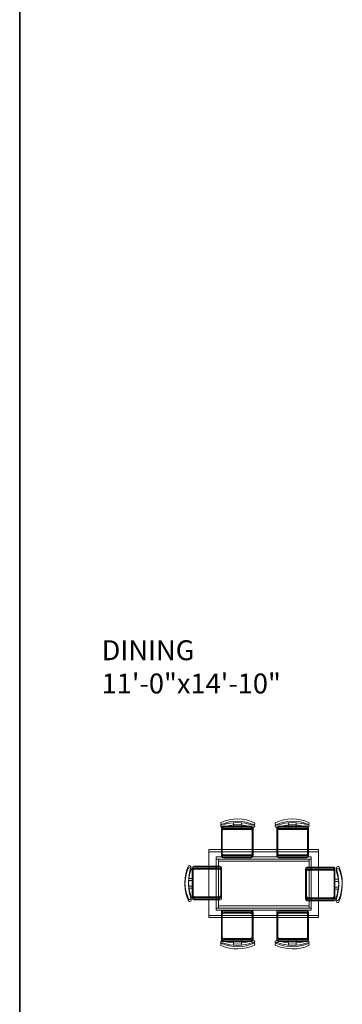
# Model space of a CAD drawing. Units: inches. Extents: x 2163 to 2982, y 1024 to 2288.
# Tile 6 of 22: x 2587 to 2668, y 1390 to 1637. Entities that reach past the tile are written whole.
import ezdxf

# ---------------------------------------------------------------- set-up
doc = ezdxf.new("R2010")
doc.units = ezdxf.units.IN
for name, color, linetype, lineweight in [('A-AREA-IDEN', 7, 'Continuous', 18), ('A-FURN', 8, 'Continuous', 13), ('A-WALL', 7, 'Continuous', 35)]:
    doc.layers.add(name, color=color, linetype=linetype, lineweight=lineweight)
doc.styles.get("Standard").update_dxf_attribs({"font": 'arial.ttf'})

# ---------------------------------------------------------------- blocks, each defined once
blk = doc.blocks.new('TABLE-DINING')
for points in [[(0, 17.02), (27.45, 17.02), (27.45, 0.55), (0, 0.55)], [(0, 17.02), (27.45, 17.02), (27.45, 0.55), (0, 0.55)], [(0, 17.02), (27.45, 17.02), (27.45, 0.55), (0, 0.55)], [(0, 17.02), (27.45, 17.02), (27.45, 0.55), (0, 0.55)], [(0, 16.47), (27.45, 16.47), (27.45, 0), (0, 0)], [(0, 16.47), (27.45, 16.47), (27.45, 0), (0, 0)], [(0, 16.47), (27.45, 16.47), (27.45, 0), (0, 0)], [(0, 16.47), (27.45, 16.47), (27.45, 0), (0, 0)], [(1.83, 15.19), (25.62, 15.19), (25.62, 2.38), (1.83, 2.38)], [(1.83, 15.19), (25.62, 15.19), (25.62, 2.38), (1.83, 2.38)], [(1.83, 15.19), (25.62, 15.19), (25.62, 2.38), (1.83, 2.38)], [(1.83, 15.19), (25.62, 15.19), (25.62, 2.38), (1.83, 2.38)], [(1.83, 14.64), (25.62, 14.64), (25.62, 1.83), (1.83, 1.83)], [(1.83, 14.64), (25.62, 14.64), (25.62, 1.83), (1.83, 1.83)], [(1.83, 14.64), (25.62, 14.64), (25.62, 1.83), (1.83, 1.83)], [(1.83, 14.64), (25.62, 14.64), (25.62, 1.83), (1.83, 1.83)], [(2.38, 14.64), (25.07, 14.64), (25.07, 2.93), (2.38, 2.93)], [(2.38, 14.64), (25.07, 14.64), (25.07, 2.93), (2.38, 2.93)], [(2.38, 14.64), (25.07, 14.64), (25.07, 2.93), (2.38, 2.93)], [(2.38, 14.64), (25.07, 14.64), (25.07, 2.93), (2.38, 2.93)], [(2.38, 14.09), (25.07, 14.09), (25.07, 2.38), (2.38, 2.38)], [(2.38, 14.09), (25.07, 14.09), (25.07, 2.38), (2.38, 2.38)], [(2.38, 14.09), (25.07, 14.09), (25.07, 2.38), (2.38, 2.38)], [(2.38, 14.09), (25.07, 14.09), (25.07, 2.38), (2.38, 2.38)]]:
    blk.add_lwpolyline(points, close=True)
blk = doc.blocks.new('CHAIR-DINING-A')
for points in [[(0.45, 8.2, -0.175809), (7.92, 8.14, 0.578392), (8.49, 8.77, 0.214524), (0.05, 8.88, 0.552014), (0.45, 8.2, -0.065079)], [(0.45, 8.2, -0.175809), (7.92, 8.14, 0.578392), (8.49, 8.77, 0.214524), (0.05, 8.88, 0.552014), (0.45, 8.2, -0.065079)], [(0.45, 8.2, -0.175809), (7.92, 8.14, 0.578392), (8.49, 8.77, 0.214524), (0.05, 8.88, 0.552014), (0.45, 8.2, -0.065079)], [(0.45, 8.2, -0.175809), (7.92, 8.14, 0.578392), (8.49, 8.77, 0.214524), (0.05, 8.88, 0.552014), (0.45, 8.2, -0.065079)], [(0.45, 7.65, -0.175809), (7.92, 7.6, 0.578392), (8.49, 8.22, 0.214524), (0.05, 8.33, 0.552014), (0.45, 7.65, -0.065079)], [(0.45, 7.65, -0.175809), (7.92, 7.6, 0.578392), (8.49, 8.22, 0.214524), (0.05, 8.33, 0.552014), (0.45, 7.65, -0.065079)], [(0.45, 7.65, -0.175809), (7.92, 7.6, 0.578392), (8.49, 8.22, 0.214524), (0.05, 8.33, 0.552014), (0.45, 7.65, -0.065079)], [(0.45, 7.65, -0.175809), (7.92, 7.6, 0.578392), (8.49, 8.22, 0.214524), (0.05, 8.33, 0.552014), (0.45, 7.65, -0.065079)], [(7.61, 7.9), (0.67, 7.9, 0.414214), (0.18, 7.42), (0.18, 1.03, 0.414214), (0.67, 0.55), (7.61, 0.55, 0.414214), (8.09, 1.03), (8.09, 7.42, 0.414214), (7.61, 7.9)], [(7.61, 7.9), (0.67, 7.9, 0.414214), (0.18, 7.42), (0.18, 1.03, 0.414214), (0.67, 0.55), (7.61, 0.55, 0.414214), (8.09, 1.03), (8.09, 7.42, 0.414214), (7.61, 7.9)], [(7.61, 7.9), (0.67, 7.9, 0.414214), (0.18, 7.42), (0.18, 1.03, 0.414214), (0.67, 0.55), (7.61, 0.55, 0.414214), (8.09, 1.03), (8.09, 7.42, 0.414214), (7.61, 7.9)], [(7.61, 7.9), (0.67, 7.9, 0.414214), (0.18, 7.42), (0.18, 1.03, 0.414214), (0.67, 0.55), (7.61, 0.55, 0.414214), (8.09, 1.03), (8.09, 7.42, 0.414214), (7.61, 7.9)], [(5.17, 7.9), (5.17, 8.78, -0.064759)], [(5.17, 7.9), (5.17, 8.78, -0.064759)], [(5.17, 7.9), (5.17, 8.78, -0.064759)], [(5.17, 7.9), (5.17, 8.78, -0.064759)], [(5.17, 7.35), (5.17, 8.23, -0.064759)], [(5.17, 7.35), (5.17, 8.23, -0.064759)], [(5.17, 7.35), (5.17, 8.23, -0.064759)], [(5.17, 7.35), (5.17, 8.23, -0.064759)], [(7.61, 7.35), (0.67, 7.35, 0.414214), (0.18, 6.87), (0.18, 0.49, 0.414214), (0.67, 0), (7.61, 0, 0.414214), (8.09, 0.49), (8.09, 6.87, 0.414214), (7.61, 7.35)], [(7.61, 7.35), (0.67, 7.35, 0.414214), (0.18, 6.87), (0.18, 0.49, 0.414214), (0.67, 0), (7.61, 0, 0.414214), (8.09, 0.49), (8.09, 6.87, 0.414214), (7.61, 7.35)], [(7.61, 7.35), (0.67, 7.35, 0.414214), (0.18, 6.87), (0.18, 0.49, 0.414214), (0.67, 0), (7.61, 0, 0.414214), (8.09, 0.49), (8.09, 6.87, 0.414214), (7.61, 7.35)], [(7.61, 7.35), (0.67, 7.35, 0.414214), (0.18, 6.87), (0.18, 0.49, 0.414214), (0.67, 0), (7.61, 0, 0.414214), (8.09, 0.49), (8.09, 6.87, 0.414214), (7.61, 7.35)]]:
    blk.add_lwpolyline(points, format="xyb")
for points in [[(0.67, 7.68), (7.39, 7.68, -0.414214), (7.87, 7.2), (7.87, 1.25, -0.414214), (7.39, 0.77), (0.67, 0.77, -0.512069), (0.4, 1.25), (0.4, 7.2, -0.512069)], [(0.67, 7.68), (7.39, 7.68, -0.414214), (7.87, 7.2), (7.87, 1.25, -0.414214), (7.39, 0.77), (0.67, 0.77, -0.512069), (0.4, 1.25), (0.4, 7.2, -0.512069)], [(0.67, 7.68), (7.39, 7.68, -0.414214), (7.87, 7.2), (7.87, 1.25, -0.414214), (7.39, 0.77), (0.67, 0.77, -0.512069), (0.4, 1.25), (0.4, 7.2, -0.512069)], [(0.67, 7.68), (7.39, 7.68, -0.414214), (7.87, 7.2), (7.87, 1.25, -0.414214), (7.39, 0.77), (0.67, 0.77, -0.512069), (0.4, 1.25), (0.4, 7.2, -0.512069)], [(0.67, 7.13), (7.39, 7.13, -0.414214), (7.87, 6.65), (7.87, 0.7, -0.414214), (7.39, 0.22), (0.67, 0.22, -0.512069), (0.4, 0.7), (0.4, 6.65, -0.512069)], [(0.67, 7.13), (7.39, 7.13, -0.414214), (7.87, 6.65), (7.87, 0.7, -0.414214), (7.39, 0.22), (0.67, 0.22, -0.512069), (0.4, 0.7), (0.4, 6.65, -0.512069)], [(0.67, 7.13), (7.39, 7.13, -0.414214), (7.87, 6.65), (7.87, 0.7, -0.414214), (7.39, 0.22), (0.67, 0.22, -0.512069), (0.4, 0.7), (0.4, 6.65, -0.512069)], [(0.67, 7.13), (7.39, 7.13, -0.414214), (7.87, 6.65), (7.87, 0.7, -0.414214), (7.39, 0.22), (0.67, 0.22, -0.512069), (0.4, 0.7), (0.4, 6.65, -0.512069)]]:
    blk.add_lwpolyline(points, format="xyb", close=True)
for points in [[(3.23, 8.8), (3.23, 7.9)], [(3.23, 8.8), (3.23, 7.9)], [(3.23, 8.79), (3.23, 7.9)], [(3.23, 8.79), (3.23, 7.9)], [(3.23, 8.25), (3.23, 7.35)], [(3.23, 8.25), (3.23, 7.35)], [(3.23, 8.25), (3.23, 7.35)], [(3.23, 8.25), (3.23, 7.35)]]:
    blk.add_lwpolyline(points)
blk = doc.blocks.new('CHAIR-DINING-B')
for points in [[(7.61, 2.38), (0.67, 2.38, -0.414214), (0.18, 2.86), (0.18, 9.24, -0.414214), (0.67, 9.73), (7.61, 9.73, -0.414214), (8.09, 9.24), (8.09, 2.86, -0.414214), (7.61, 2.38)], [(7.61, 2.38), (0.67, 2.38, -0.414214), (0.18, 2.86), (0.18, 9.24, -0.414214), (0.67, 9.73), (7.61, 9.73, -0.414214), (8.09, 9.24), (8.09, 2.86, -0.414214), (7.61, 2.38)], [(7.61, 2.38), (0.67, 2.38, -0.414214), (0.18, 2.86), (0.18, 9.24, -0.414214), (0.67, 9.73), (7.61, 9.73, -0.414214), (8.09, 9.24), (8.09, 2.86, -0.414214), (7.61, 2.38)], [(7.61, 2.38), (0.67, 2.38, -0.414214), (0.18, 2.86), (0.18, 9.24, -0.414214), (0.67, 9.73), (7.61, 9.73, -0.414214), (8.09, 9.24), (8.09, 2.86, -0.414214), (7.61, 2.38)], [(7.61, 1.83), (0.67, 1.83, -0.414214), (0.18, 2.31), (0.18, 8.69, -0.414214), (0.67, 9.18), (7.61, 9.18, -0.414214), (8.09, 8.69), (8.09, 2.31, -0.414214), (7.61, 1.83)], [(7.61, 1.83), (0.67, 1.83, -0.414214), (0.18, 2.31), (0.18, 8.69, -0.414214), (0.67, 9.18), (7.61, 9.18, -0.414214), (8.09, 8.69), (8.09, 2.31, -0.414214), (7.61, 1.83)], [(7.61, 1.83), (0.67, 1.83, -0.414214), (0.18, 2.31), (0.18, 8.69, -0.414214), (0.67, 9.18), (7.61, 9.18, -0.414214), (8.09, 8.69), (8.09, 2.31, -0.414214), (7.61, 1.83)], [(7.61, 1.83), (0.67, 1.83, -0.414214), (0.18, 2.31), (0.18, 8.69, -0.414214), (0.67, 9.18), (7.61, 9.18, -0.414214), (8.09, 8.69), (8.09, 2.31, -0.414214), (7.61, 1.83)], [(7.92, 2.13, -0.578392), (8.49, 1.51, -0.214524), (0.05, 1.4, -0.552014), (0.45, 2.08, 0.175809), (7.92, 2.13)], [(7.92, 2.13, -0.578392), (8.49, 1.51, -0.214524), (0.05, 1.4, -0.552014), (0.45, 2.08, 0.175809), (7.92, 2.13)], [(7.92, 2.13, -0.578392), (8.49, 1.51, -0.214524), (0.05, 1.4, -0.552014), (0.45, 2.08, 0.175809), (7.92, 2.13)], [(7.92, 2.13, -0.578392), (8.49, 1.51, -0.214524), (0.05, 1.4, -0.552014), (0.45, 2.08, 0.175809), (7.92, 2.13)], [(7.92, 1.58, -0.578392), (8.49, 0.96, -0.214524), (0.05, 0.85, -0.552014), (0.45, 1.53, 0.175809), (7.92, 1.58)], [(7.92, 1.58, -0.578392), (8.49, 0.96, -0.214524), (0.05, 0.85, -0.552014), (0.45, 1.53, 0.175809), (7.92, 1.58)], [(7.92, 1.58, -0.578392), (8.49, 0.96, -0.214524), (0.05, 0.85, -0.552014), (0.45, 1.53, 0.175809), (7.92, 1.58)], [(7.92, 1.58, -0.578392), (8.49, 0.96, -0.214524), (0.05, 0.85, -0.552014), (0.45, 1.53, 0.175809), (7.92, 1.58)], [(5.17, 2.38), (5.17, 1.5, 0.064759)], [(5.17, 2.38), (5.17, 1.5, 0.064759)], [(5.17, 2.38), (5.17, 1.5, 0.064759)], [(5.17, 2.38), (5.17, 1.5, 0.064759)], [(5.17, 1.83), (5.17, 0.95, 0.064759)], [(5.17, 1.83), (5.17, 0.95, 0.064759)], [(5.17, 1.83), (5.17, 0.95, 0.064759)], [(5.17, 1.83), (5.17, 0.95, 0.064759)]]:
    blk.add_lwpolyline(points, format="xyb")
for points in [[(0.67, 2.6), (7.39, 2.6, 0.414214), (7.87, 3.08), (7.87, 9.02, 0.414214), (7.39, 9.51), (0.67, 9.51, 0.512069), (0.4, 9.02), (0.4, 3.08, 0.512069)], [(0.67, 2.6), (7.39, 2.6, 0.414214), (7.87, 3.08), (7.87, 9.02, 0.414214), (7.39, 9.51), (0.67, 9.51, 0.512069), (0.4, 9.02), (0.4, 3.08, 0.512069)], [(0.67, 2.6), (7.39, 2.6, 0.414214), (7.87, 3.08), (7.87, 9.02, 0.414214), (7.39, 9.51), (0.67, 9.51, 0.512069), (0.4, 9.02), (0.4, 3.08, 0.512069)], [(0.67, 2.6), (7.39, 2.6, 0.414214), (7.87, 3.08), (7.87, 9.02, 0.414214), (7.39, 9.51), (0.67, 9.51, 0.512069), (0.4, 9.02), (0.4, 3.08, 0.512069)], [(0.67, 2.05), (7.39, 2.05, 0.414214), (7.87, 2.53), (7.87, 8.48, 0.414214), (7.39, 8.96), (0.67, 8.96, 0.512069), (0.4, 8.48), (0.4, 2.53, 0.512069)], [(0.67, 2.05), (7.39, 2.05, 0.414214), (7.87, 2.53), (7.87, 8.48, 0.414214), (7.39, 8.96), (0.67, 8.96, 0.512069), (0.4, 8.48), (0.4, 2.53, 0.512069)], [(0.67, 2.05), (7.39, 2.05, 0.414214), (7.87, 2.53), (7.87, 8.48, 0.414214), (7.39, 8.96), (0.67, 8.96, 0.512069), (0.4, 8.48), (0.4, 2.53, 0.512069)], [(0.67, 2.05), (7.39, 2.05, 0.414214), (7.87, 2.53), (7.87, 8.48, 0.414214), (7.39, 8.96), (0.67, 8.96, 0.512069), (0.4, 8.48), (0.4, 2.53, 0.512069)]]:
    blk.add_lwpolyline(points, format="xyb", close=True)
for points in [[(3.23, 1.48), (3.23, 2.38)], [(3.23, 1.48), (3.23, 2.38)], [(3.23, 1.48), (3.23, 2.38)], [(3.23, 1.48), (3.23, 2.38)], [(3.23, 0.93), (3.23, 1.83)], [(3.23, 0.93), (3.23, 1.83)], [(3.23, 0.93), (3.23, 1.83)], [(3.23, 0.93), (3.23, 1.83)]]:
    blk.add_lwpolyline(points)

msp = doc.modelspace()

# ---------------------------------------------------------------- linework, layer by layer
at = {"layer": 'A-FURN'}
for points in [[(2651.3919, 1435.1979, -0.57839206), (2650.8255, 1435.8207, -0.21452438), (2659.2637, 1435.9339, -0.55201397), (2658.8673, 1435.2546, 0.1758092), (2651.3919, 1435.1979)], [(2651.3919, 1435.1979, -0.57839206), (2650.8255, 1435.8207, -0.21452438), (2659.2637, 1435.9339, -0.55201397), (2658.8673, 1435.2546, 0.1758092), (2651.3919, 1435.1979)], [(2651.3919, 1435.1977, -0.57839206), (2650.8255, 1435.8204, -0.21452438), (2659.2637, 1435.9336, -0.55201397), (2658.8673, 1435.2543, 0.1758092), (2651.3919, 1435.1977)], [(2651.3919, 1435.1977, -0.57839206), (2650.8255, 1435.8204, -0.21452438), (2659.2637, 1435.9336, -0.55201397), (2658.8673, 1435.2543, 0.1758092), (2651.3919, 1435.1977)], [(2651.3919, 1434.649, -0.57839206), (2650.8255, 1435.2717, -0.21452438), (2659.2637, 1435.385, -0.55201397), (2658.8673, 1434.7056, 0.1758092), (2651.3919, 1434.649)], [(2651.3919, 1434.649, -0.57839206), (2650.8255, 1435.2717, -0.21452438), (2659.2637, 1435.385, -0.55201397), (2658.8673, 1434.7056, 0.1758092), (2651.3919, 1434.649)], [(2651.3919, 1434.6487, -0.57839206), (2650.8255, 1435.2715, -0.21452438), (2659.2637, 1435.3847, -0.55201397), (2658.8673, 1434.7053, 0.1758092), (2651.3919, 1434.6487)], [(2651.3919, 1434.6487, -0.57839206), (2650.8255, 1435.2715, -0.21452438), (2659.2637, 1435.3847, -0.55201397), (2658.8673, 1434.7053, 0.1758092), (2651.3919, 1434.6487)], [(2658.6489, 1434.9545, -0.41421356), (2659.1345, 1434.469), (2659.1345, 1428.0879, -0.41421356), (2658.6489, 1427.6023), (2651.709, 1427.6023, -0.41421356), (2651.2235, 1428.0879), (2651.2235, 1434.469, -0.41421356), (2651.709, 1434.9545), (2658.6489, 1434.9545)], [(2658.6489, 1434.9545, -0.41421356), (2659.1345, 1434.469), (2659.1345, 1428.0879, -0.41421356), (2658.6489, 1427.6023), (2651.709, 1427.6023, -0.41421356), (2651.2235, 1428.0879), (2651.2235, 1434.469, -0.41421356), (2651.709, 1434.9545), (2658.6489, 1434.9545)], [(2658.649, 1434.9542, -0.41421356), (2659.1345, 1434.4687), (2659.1345, 1428.0876, -0.41421356), (2658.649, 1427.602), (2651.709, 1427.602, -0.41421356), (2651.2235, 1428.0876), (2651.2235, 1434.4687, -0.41421356), (2651.709, 1434.9542), (2658.649, 1434.9542)], [(2658.649, 1434.9542, -0.41421356), (2659.1345, 1434.4687), (2659.1345, 1428.0876, -0.41421356), (2658.649, 1427.602), (2651.709, 1427.602, -0.41421356), (2651.2235, 1428.0876), (2651.2235, 1434.4687, -0.41421356), (2651.709, 1434.9542), (2658.649, 1434.9542)], [(2658.6489, 1434.4056, -0.41421356), (2659.1345, 1433.9201), (2659.1345, 1427.5389, -0.41421356), (2658.6489, 1427.0534), (2651.709, 1427.0534, -0.41421356), (2651.2235, 1427.5389), (2651.2235, 1433.9201, -0.41421356), (2651.709, 1434.4056), (2658.6489, 1434.4056)], [(2658.6489, 1434.4056, -0.41421356), (2659.1345, 1433.9201), (2659.1345, 1427.5389, -0.41421356), (2658.6489, 1427.0534), (2651.709, 1427.0534, -0.41421356), (2651.2235, 1427.5389), (2651.2235, 1433.9201, -0.41421356), (2651.709, 1434.4056), (2658.6489, 1434.4056)], [(2658.649, 1434.4053, -0.41421356), (2659.1345, 1433.9198), (2659.1345, 1427.5386, -0.41421356), (2658.649, 1427.0531), (2651.709, 1427.0531, -0.41421356), (2651.2235, 1427.5386), (2651.2235, 1433.9198, -0.41421356), (2651.709, 1434.4053), (2658.649, 1434.4053)], [(2658.649, 1434.4053, -0.41421356), (2659.1345, 1433.9198), (2659.1345, 1427.5386, -0.41421356), (2658.649, 1427.0531), (2651.709, 1427.0531, -0.41421356), (2651.2235, 1427.5386), (2651.2235, 1433.9198, -0.41421356), (2651.709, 1434.4053), (2658.649, 1434.4053)], [(2654.1467, 1434.9545), (2654.1467, 1435.8322, 0.06475861)], [(2654.1467, 1434.9545), (2654.1467, 1435.8322, 0.06475861)], [(2654.1467, 1434.9542), (2654.1467, 1435.8319, 0.06475861)], [(2654.1467, 1434.9542), (2654.1467, 1435.8319, 0.06475861)], [(2654.1467, 1434.4056), (2654.1467, 1435.2833, 0.06475861)], [(2654.1467, 1434.4056), (2654.1467, 1435.2833, 0.06475861)], [(2654.1467, 1434.4053), (2654.1467, 1435.283, 0.06475861)], [(2654.1467, 1434.4053), (2654.1467, 1435.283, 0.06475861)], [(2629.8023, 1417.2025, -0.57839206), (2629.1796, 1416.6362, -0.21452438), (2629.0664, 1425.0744, -0.55201397), (2629.7457, 1424.6779, 0.17580937), (2629.8023, 1417.2025)], [(2629.8023, 1417.2025, -0.57839206), (2629.1796, 1416.6362, -0.21452438), (2629.0664, 1425.0744, -0.55201397), (2629.7457, 1424.6779, 0.17580937), (2629.8023, 1417.2025)], [(2629.8023, 1417.2022, -0.57839206), (2629.1796, 1416.6359, -0.21452438), (2629.0664, 1425.0741, -0.55201397), (2629.7457, 1424.6777, 0.17580937), (2629.8023, 1417.2022)], [(2629.8023, 1417.2022, -0.57839206), (2629.1796, 1416.6359, -0.21452438), (2629.0664, 1425.0741, -0.55201397), (2629.7457, 1424.6777, 0.17580937), (2629.8023, 1417.2022)], [(2629.8023, 1416.6536, -0.57839206), (2629.1796, 1416.0873, -0.21452438), (2629.0664, 1424.5255, -0.55201397), (2629.7457, 1424.129, 0.17580937), (2629.8023, 1416.6536)], [(2629.8023, 1416.6536, -0.57839206), (2629.1796, 1416.0873, -0.21452438), (2629.0664, 1424.5255, -0.55201397), (2629.7457, 1424.129, 0.17580937), (2629.8023, 1416.6536)], [(2629.8023, 1416.6533, -0.57839206), (2629.1796, 1416.087, -0.21452438), (2629.0664, 1424.5252, -0.55201397), (2629.7457, 1424.1287, 0.17580937), (2629.8023, 1416.6533)], [(2629.8023, 1416.6533, -0.57839206), (2629.1796, 1416.087, -0.21452438), (2629.0664, 1424.5252, -0.55201397), (2629.7457, 1424.1287, 0.17580937), (2629.8023, 1416.6533)], [(2630.0457, 1424.4596, -0.41421356), (2630.5313, 1424.9451), (2636.9124, 1424.9451, -0.41421356), (2637.3979, 1424.4596), (2637.3979, 1417.5197, -0.41421356), (2636.9124, 1417.0341), (2630.5313, 1417.0341, -0.41421356), (2630.0457, 1417.5197), (2630.0457, 1424.4596)], [(2630.0457, 1424.4596, -0.41421356), (2630.5313, 1424.9451), (2636.9124, 1424.9451, -0.41421356), (2637.3979, 1424.4596), (2637.3979, 1417.5197, -0.41421356), (2636.9124, 1417.0341), (2630.5313, 1417.0341, -0.41421356), (2630.0457, 1417.5197), (2630.0457, 1424.4596)], [(2630.0457, 1423.9107, -0.41421356), (2630.5313, 1424.3962), (2636.9124, 1424.3962, -0.41421356), (2637.3979, 1423.9107), (2637.3979, 1416.9707, -0.41421356), (2636.9124, 1416.4852), (2630.5313, 1416.4852, -0.41421356), (2630.0457, 1416.9707), (2630.0457, 1423.9107)], [(2630.0457, 1423.9107, -0.41421356), (2630.5313, 1424.3962), (2636.9124, 1424.3962, -0.41421356), (2637.3979, 1423.9107), (2637.3979, 1416.9707, -0.41421356), (2636.9124, 1416.4852), (2630.5313, 1416.4852, -0.41421356), (2630.0457, 1416.9707), (2630.0457, 1423.9107)], [(2630.0458, 1424.4593, -0.41421356), (2630.5313, 1424.9448), (2636.9124, 1424.9448, -0.41421356), (2637.3979, 1424.4593), (2637.3979, 1417.5194, -0.41421356), (2636.9124, 1417.0338), (2630.5313, 1417.0338, -0.41421356), (2630.0458, 1417.5194), (2630.0458, 1424.4593)], [(2630.0458, 1424.4593, -0.41421356), (2630.5313, 1424.9448), (2636.9124, 1424.9448, -0.41421356), (2637.3979, 1424.4593), (2637.3979, 1417.5194, -0.41421356), (2636.9124, 1417.0338), (2630.5313, 1417.0338, -0.41421356), (2630.0458, 1417.5194), (2630.0458, 1424.4593)], [(2630.0458, 1423.9104, -0.41421356), (2630.5313, 1424.3959), (2636.9124, 1424.3959, -0.41421356), (2637.3979, 1423.9104), (2637.3979, 1416.9705, -0.41421356), (2636.9124, 1416.4849), (2630.5313, 1416.4849, -0.41421356), (2630.0458, 1416.9705), (2630.0458, 1423.9104)], [(2630.0458, 1423.9104, -0.41421356), (2630.5313, 1424.3959), (2636.9124, 1424.3959, -0.41421356), (2637.3979, 1423.9104), (2637.3979, 1416.9705, -0.41421356), (2636.9124, 1416.4849), (2630.5313, 1416.4849, -0.41421356), (2630.0458, 1416.9705), (2630.0458, 1423.9104)], [(2665.7832, 1424.2219, 0.41421356), (2665.2977, 1424.7074), (2658.9165, 1424.7074, 0.41421356), (2658.431, 1424.2219), (2658.431, 1417.282, 0.41421356), (2658.9165, 1416.7965), (2665.2977, 1416.7965, 0.41421356), (2665.7832, 1417.282), (2665.7832, 1424.2219)], [(2665.7832, 1424.2219, 0.41421356), (2665.2977, 1424.7074), (2658.9165, 1424.7074, 0.41421356), (2658.431, 1424.2219), (2658.431, 1417.282, 0.41421356), (2658.9165, 1416.7965), (2665.2977, 1416.7965, 0.41421356), (2665.7832, 1417.282), (2665.7832, 1424.2219)], [(2665.7832, 1424.2216, 0.41421356), (2665.2977, 1424.7072), (2658.9165, 1424.7072, 0.41421356), (2658.431, 1424.2216), (2658.431, 1417.2817, 0.41421356), (2658.9165, 1416.7962), (2665.2977, 1416.7962, 0.41421356), (2665.7832, 1417.2817), (2665.7832, 1424.2216)], [(2665.7832, 1424.2216, 0.41421356), (2665.2977, 1424.7072), (2658.9165, 1424.7072, 0.41421356), (2658.431, 1424.2216), (2658.431, 1417.2817, 0.41421356), (2658.9165, 1416.7962), (2665.2977, 1416.7962, 0.41421356), (2665.7832, 1417.2817), (2665.7832, 1424.2216)], [(2665.7832, 1423.673, 0.41421356), (2665.2977, 1424.1585), (2658.9165, 1424.1585, 0.41421356), (2658.431, 1423.673), (2658.431, 1416.7331, 0.41421356), (2658.9165, 1416.2475), (2665.2977, 1416.2475, 0.41421356), (2665.7832, 1416.7331), (2665.7832, 1423.673)], [(2665.7832, 1423.673, 0.41421356), (2665.2977, 1424.1585), (2658.9165, 1424.1585, 0.41421356), (2658.431, 1423.673), (2658.431, 1416.7331, 0.41421356), (2658.9165, 1416.2475), (2665.2977, 1416.2475, 0.41421356), (2665.7832, 1416.7331), (2665.7832, 1423.673)], [(2665.7832, 1423.6727, 0.41421356), (2665.2977, 1424.1582), (2658.9165, 1424.1582, 0.41421356), (2658.431, 1423.6727), (2658.431, 1416.7328, 0.41421356), (2658.9165, 1416.2472), (2665.2977, 1416.2472, 0.41421356), (2665.7832, 1416.7328), (2665.7832, 1423.6727)], [(2665.7832, 1423.6727, 0.41421356), (2665.2977, 1424.1582), (2658.9165, 1424.1582, 0.41421356), (2658.431, 1423.6727), (2658.431, 1416.7328, 0.41421356), (2658.9165, 1416.2472), (2665.2977, 1416.2472, 0.41421356), (2665.7832, 1416.7328), (2665.7832, 1423.6727)], [(2666.0832, 1424.4403, -0.17580919), (2666.0266, 1416.9648, 0.57839206), (2666.6493, 1416.3985, 0.21452438), (2666.7626, 1424.8367, 0.55201397), (2666.0832, 1424.4403, -0.06507904)], [(2666.0832, 1424.4403, -0.17580919), (2666.0266, 1416.9648, 0.57839206), (2666.6493, 1416.3985, 0.21452438), (2666.7626, 1424.8367, 0.55201397), (2666.0832, 1424.4403, -0.06507904)], [(2666.0832, 1423.8913, -0.17580919), (2666.0266, 1416.4159, 0.57839206), (2666.6493, 1415.8496, 0.21452438), (2666.7626, 1424.2878, 0.55201397), (2666.0832, 1423.8914, -0.06507904)], [(2666.0832, 1423.8913, -0.17580919), (2666.0266, 1416.4159, 0.57839206), (2666.6493, 1415.8496, 0.21452438), (2666.7626, 1424.2878, 0.55201397), (2666.0832, 1423.8914, -0.06507904)], [(2666.0832, 1424.44, -0.17580919), (2666.0266, 1416.9645, 0.57839206), (2666.6493, 1416.3982, 0.21452438), (2666.7626, 1424.8364, 0.55201397), (2666.0832, 1424.44, -0.06507904)], [(2666.0832, 1424.44, -0.17580919), (2666.0266, 1416.9645, 0.57839206), (2666.6493, 1416.3982, 0.21452438), (2666.7626, 1424.8364, 0.55201397), (2666.0832, 1424.44, -0.06507904)], [(2666.0832, 1423.8911, -0.17580919), (2666.0266, 1416.4156, 0.57839206), (2666.6493, 1415.8493, 0.21452438), (2666.7626, 1424.2875, 0.55201397), (2666.0832, 1423.8911, -0.06507904)], [(2666.0832, 1423.8911, -0.17580919), (2666.0266, 1416.4156, 0.57839206), (2666.6493, 1415.8493, 0.21452438), (2666.7626, 1424.2875, 0.55201397), (2666.0832, 1423.8911, -0.06507904)], [(2630.0457, 1419.9573), (2629.168, 1419.9573, 0.06475861)], [(2630.0457, 1419.9573), (2629.168, 1419.9573, 0.06475861)], [(2630.0457, 1419.4084), (2629.168, 1419.4084, 0.06475861)], [(2630.0457, 1419.4084), (2629.168, 1419.4084, 0.06475861)], [(2630.0458, 1419.957), (2629.1681, 1419.957, 0.06475861)], [(2630.0458, 1419.957), (2629.1681, 1419.957, 0.06475861)], [(2630.0458, 1419.4081), (2629.1681, 1419.4081, 0.06475861)], [(2630.0458, 1419.4081), (2629.1681, 1419.4081, 0.06475861)], [(2665.7832, 1419.7196), (2666.6609, 1419.7196, -0.06475861)], [(2665.7832, 1419.7196), (2666.6609, 1419.7196, -0.06475861)], [(2665.7832, 1419.7193), (2666.6609, 1419.7193, -0.06475861)], [(2665.7832, 1419.7193), (2666.6609, 1419.7193, -0.06475861)], [(2665.7832, 1419.1707), (2666.6609, 1419.1707, -0.06475861)], [(2665.7832, 1419.1707), (2666.6609, 1419.1707, -0.06475861)], [(2665.7832, 1419.1704), (2666.6609, 1419.1704, -0.06475861)], [(2665.7832, 1419.1704), (2666.6609, 1419.1704, -0.06475861)], [(2658.6489, 1406.5888, 0.41421356), (2659.1345, 1407.0743), (2659.1345, 1413.4554, 0.41421356), (2658.6489, 1413.941), (2651.709, 1413.941, 0.41421356), (2651.2235, 1413.4554), (2651.2235, 1407.0743, 0.41421356), (2651.709, 1406.5888), (2658.6489, 1406.5888)], [(2658.6489, 1406.5888, 0.41421356), (2659.1345, 1407.0743), (2659.1345, 1413.4554, 0.41421356), (2658.6489, 1413.941), (2651.709, 1413.941, 0.41421356), (2651.2235, 1413.4554), (2651.2235, 1407.0743, 0.41421356), (2651.709, 1406.5888), (2658.6489, 1406.5888)], [(2658.649, 1406.5885, 0.41421356), (2659.1345, 1407.074), (2659.1345, 1413.4552, 0.41421356), (2658.649, 1413.9407), (2651.709, 1413.9407, 0.41421356), (2651.2235, 1413.4552), (2651.2235, 1407.074, 0.41421356), (2651.709, 1406.5885), (2658.649, 1406.5885)], [(2658.649, 1406.5885, 0.41421356), (2659.1345, 1407.074), (2659.1345, 1413.4552, 0.41421356), (2658.649, 1413.9407), (2651.709, 1413.9407, 0.41421356), (2651.2235, 1413.4552), (2651.2235, 1407.074, 0.41421356), (2651.709, 1406.5885), (2658.649, 1406.5885)], [(2658.6489, 1406.0399, 0.41421356), (2659.1345, 1406.5254), (2659.1345, 1412.9065, 0.41421356), (2658.6489, 1413.3921), (2651.709, 1413.3921, 0.41421356), (2651.2235, 1412.9065), (2651.2235, 1406.5254, 0.41421356), (2651.709, 1406.0399), (2658.6489, 1406.0399)], [(2658.6489, 1406.0399, 0.41421356), (2659.1345, 1406.5254), (2659.1345, 1412.9065, 0.41421356), (2658.6489, 1413.3921), (2651.709, 1413.3921, 0.41421356), (2651.2235, 1412.9065), (2651.2235, 1406.5254, 0.41421356), (2651.709, 1406.0399), (2658.6489, 1406.0399)], [(2658.649, 1406.0396, 0.41421356), (2659.1345, 1406.5251), (2659.1345, 1412.9062, 0.41421356), (2658.649, 1413.3918), (2651.709, 1413.3918, 0.41421356), (2651.2235, 1412.9062), (2651.2235, 1406.5251, 0.41421356), (2651.709, 1406.0396), (2658.649, 1406.0396)], [(2658.649, 1406.0396, 0.41421356), (2659.1345, 1406.5251), (2659.1345, 1412.9062, 0.41421356), (2658.649, 1413.3918), (2651.709, 1413.3918, 0.41421356), (2651.2235, 1412.9062), (2651.2235, 1406.5251, 0.41421356), (2651.709, 1406.0396), (2658.649, 1406.0396)], [(2658.8673, 1406.2887, -0.17580928), (2651.3919, 1406.3454, 0.57839206), (2650.8255, 1405.7226, 0.21452438), (2659.2637, 1405.6094, 0.55201397), (2658.8673, 1406.2887, -0.06507904)], [(2658.8673, 1406.2887, -0.17580928), (2651.3919, 1406.3454, 0.57839206), (2650.8255, 1405.7226, 0.21452438), (2659.2637, 1405.6094, 0.55201397), (2658.8673, 1406.2887, -0.06507904)], [(2658.8673, 1406.2885, -0.17580928), (2651.3919, 1406.3451, 0.57839206), (2650.8255, 1405.7224, 0.21452438), (2659.2637, 1405.6091, 0.55201397), (2658.8673, 1406.2885, -0.06507904)], [(2658.8673, 1406.2885, -0.17580928), (2651.3919, 1406.3451, 0.57839206), (2650.8255, 1405.7224, 0.21452438), (2659.2637, 1405.6091, 0.55201397), (2658.8673, 1406.2885, -0.06507904)], [(2658.8673, 1405.7398, -0.17580928), (2651.3919, 1405.7964, 0.57839206), (2650.8255, 1405.1737, 0.21452438), (2659.2637, 1405.0605, 0.55201397), (2658.8673, 1405.7398, -0.06507904)], [(2658.8673, 1405.7398, -0.17580928), (2651.3919, 1405.7964, 0.57839206), (2650.8255, 1405.1737, 0.21452438), (2659.2637, 1405.0605, 0.55201397), (2658.8673, 1405.7398, -0.06507904)], [(2658.8673, 1405.7395, -0.17580928), (2651.3919, 1405.7962, 0.57839206), (2650.8255, 1405.1734, 0.21452438), (2659.2637, 1405.0602, 0.55201397), (2658.8673, 1405.7395, -0.06507904)], [(2658.8673, 1405.7395, -0.17580928), (2651.3919, 1405.7962, 0.57839206), (2650.8255, 1405.1734, 0.21452438), (2659.2637, 1405.0602, 0.55201397), (2658.8673, 1405.7395, -0.06507904)], [(2654.1467, 1406.5888), (2654.1467, 1405.7111, -0.06475861)], [(2654.1467, 1406.5888), (2654.1467, 1405.7111, -0.06475861)], [(2654.1467, 1406.5885), (2654.1467, 1405.7108, -0.06475861)], [(2654.1467, 1406.5885), (2654.1467, 1405.7108, -0.06475861)], [(2654.1467, 1406.0399), (2654.1467, 1405.1622, -0.06475861)], [(2654.1467, 1406.0399), (2654.1467, 1405.1622, -0.06475861)], [(2654.1467, 1406.0396), (2654.1467, 1405.1619, -0.06475861)], [(2654.1467, 1406.0396), (2654.1467, 1405.1619, -0.06475861)]]:
    msp.add_lwpolyline(points, format="xyb", dxfattribs=at)
for points in [[(2658.646, 1434.7358), (2651.9277, 1434.7358, 0.41421356), (2651.4422, 1434.2503), (2651.4422, 1428.3066, 0.41421356), (2651.9277, 1427.8211), (2658.646, 1427.8211, 0.51206948), (2658.9157, 1428.3066), (2658.9157, 1434.2503, 0.51206948)], [(2658.646, 1434.7358), (2651.9277, 1434.7358, 0.41421356), (2651.4422, 1434.2503), (2651.4422, 1428.3066, 0.41421356), (2651.9277, 1427.8211), (2658.646, 1427.8211, 0.51206948), (2658.9157, 1428.3066), (2658.9157, 1434.2503, 0.51206948)], [(2658.646, 1434.7355), (2651.9277, 1434.7355, 0.41421356), (2651.4422, 1434.25), (2651.4422, 1428.3063, 0.41421356), (2651.9277, 1427.8208), (2658.646, 1427.8208, 0.51206948), (2658.9158, 1428.3063), (2658.9158, 1434.25, 0.51206948)], [(2658.646, 1434.7355), (2651.9277, 1434.7355, 0.41421356), (2651.4422, 1434.25), (2651.4422, 1428.3063, 0.41421356), (2651.9277, 1427.8208), (2658.646, 1427.8208, 0.51206948), (2658.9158, 1428.3063), (2658.9158, 1434.25, 0.51206948)], [(2658.646, 1434.1869), (2651.9277, 1434.1869, 0.41421356), (2651.4422, 1433.7014), (2651.4422, 1427.7577, 0.41421356), (2651.9277, 1427.2721), (2658.646, 1427.2721, 0.51206948), (2658.9157, 1427.7577), (2658.9157, 1433.7014, 0.51206948)], [(2658.646, 1434.1869), (2651.9277, 1434.1869, 0.41421356), (2651.4422, 1433.7014), (2651.4422, 1427.7577, 0.41421356), (2651.9277, 1427.2721), (2658.646, 1427.2721, 0.51206948), (2658.9157, 1427.7577), (2658.9157, 1433.7014, 0.51206948)], [(2658.646, 1434.1866), (2651.9277, 1434.1866, 0.41421356), (2651.4422, 1433.7011), (2651.4422, 1427.7574, 0.41421356), (2651.9277, 1427.2719), (2658.646, 1427.2719, 0.51206948), (2658.9158, 1427.7574), (2658.9158, 1433.7011, 0.51206948)], [(2658.646, 1434.1866), (2651.9277, 1434.1866, 0.41421356), (2651.4422, 1433.7011), (2651.4422, 1427.7574, 0.41421356), (2651.9277, 1427.2719), (2658.646, 1427.2719, 0.51206948), (2658.9158, 1427.7574), (2658.9158, 1433.7011, 0.51206948)], [(2630.2645, 1424.4567), (2630.2645, 1417.7384, 0.41421356), (2630.75, 1417.2529), (2636.6937, 1417.2529, 0.41421356), (2637.1792, 1417.7384), (2637.1792, 1424.4567, 0.51206948), (2636.6937, 1424.7264), (2630.75, 1424.7264, 0.51206948)], [(2630.2645, 1424.4567), (2630.2645, 1417.7384, 0.41421356), (2630.75, 1417.2529), (2636.6937, 1417.2529, 0.41421356), (2637.1792, 1417.7384), (2637.1792, 1424.4567, 0.51206948), (2636.6937, 1424.7264), (2630.75, 1424.7264, 0.51206948)], [(2630.2645, 1424.4564), (2630.2645, 1417.7381, 0.41421356), (2630.75, 1417.2526), (2636.6937, 1417.2526, 0.41421356), (2637.1792, 1417.7381), (2637.1792, 1424.4564, 0.51206948), (2636.6937, 1424.7261), (2630.75, 1424.7261, 0.51206948)], [(2630.2645, 1424.4564), (2630.2645, 1417.7381, 0.41421356), (2630.75, 1417.2526), (2636.6937, 1417.2526, 0.41421356), (2637.1792, 1417.7381), (2637.1792, 1424.4564, 0.51206948), (2636.6937, 1424.7261), (2630.75, 1424.7261, 0.51206948)], [(2630.2645, 1423.9077), (2630.2645, 1417.1895, 0.41421356), (2630.75, 1416.7039), (2636.6937, 1416.7039, 0.41421356), (2637.1792, 1417.1895), (2637.1792, 1423.9077, 0.51206948), (2636.6937, 1424.1775), (2630.75, 1424.1775, 0.51206948)], [(2630.2645, 1423.9077), (2630.2645, 1417.1895, 0.41421356), (2630.75, 1416.7039), (2636.6937, 1416.7039, 0.41421356), (2637.1792, 1417.1895), (2637.1792, 1423.9077, 0.51206948), (2636.6937, 1424.1775), (2630.75, 1424.1775, 0.51206948)], [(2630.2645, 1423.9075), (2630.2645, 1417.1892, 0.41421356), (2630.75, 1416.7037), (2636.6937, 1416.7037, 0.41421356), (2637.1792, 1417.1892), (2637.1792, 1423.9075, 0.51206948), (2636.6937, 1424.1772), (2630.75, 1424.1772, 0.51206948)], [(2630.2645, 1423.9075), (2630.2645, 1417.1892, 0.41421356), (2630.75, 1416.7037), (2636.6937, 1416.7037, 0.41421356), (2637.1792, 1417.1892), (2637.1792, 1423.9075, 0.51206948), (2636.6937, 1424.1772), (2630.75, 1424.1772, 0.51206948)], [(2665.5645, 1424.219), (2665.5645, 1417.5007, -0.41421356), (2665.0789, 1417.0152), (2659.1353, 1417.0152, -0.41421356), (2658.6497, 1417.5007), (2658.6497, 1424.219, -0.51206948), (2659.1353, 1424.4887), (2665.0789, 1424.4887, -0.51206948)], [(2665.5645, 1424.219), (2665.5645, 1417.5007, -0.41421356), (2665.0789, 1417.0152), (2659.1353, 1417.0152, -0.41421356), (2658.6497, 1417.5007), (2658.6497, 1424.219, -0.51206948), (2659.1353, 1424.4887), (2665.0789, 1424.4887, -0.51206948)], [(2665.5645, 1424.2187), (2665.5645, 1417.5004, -0.41421356), (2665.079, 1417.0149), (2659.1353, 1417.0149, -0.41421356), (2658.6497, 1417.5004), (2658.6497, 1424.2187, -0.51206948), (2659.1353, 1424.4884), (2665.079, 1424.4884, -0.51206948)], [(2665.5645, 1424.2187), (2665.5645, 1417.5004, -0.41421356), (2665.079, 1417.0149), (2659.1353, 1417.0149, -0.41421356), (2658.6497, 1417.5004), (2658.6497, 1424.2187, -0.51206948), (2659.1353, 1424.4884), (2665.079, 1424.4884, -0.51206948)], [(2665.5645, 1423.6701), (2665.5645, 1416.9518, -0.41421356), (2665.0789, 1416.4663), (2659.1353, 1416.4663, -0.41421356), (2658.6497, 1416.9518), (2658.6497, 1423.6701, -0.51206948), (2659.1353, 1423.9398), (2665.0789, 1423.9398, -0.51206948)], [(2665.5645, 1423.6701), (2665.5645, 1416.9518, -0.41421356), (2665.0789, 1416.4663), (2659.1353, 1416.4663, -0.41421356), (2658.6497, 1416.9518), (2658.6497, 1423.6701, -0.51206948), (2659.1353, 1423.9398), (2665.0789, 1423.9398, -0.51206948)], [(2665.5645, 1423.6698), (2665.5645, 1416.9515, -0.41421356), (2665.079, 1416.466), (2659.1353, 1416.466, -0.41421356), (2658.6497, 1416.9515), (2658.6497, 1423.6698, -0.51206948), (2659.1353, 1423.9395), (2665.079, 1423.9395, -0.51206948)], [(2665.5645, 1423.6698), (2665.5645, 1416.9515, -0.41421356), (2665.079, 1416.466), (2659.1353, 1416.466, -0.41421356), (2658.6497, 1416.9515), (2658.6497, 1423.6698, -0.51206948), (2659.1353, 1423.9395), (2665.079, 1423.9395, -0.51206948)], [(2658.646, 1406.8075), (2651.9277, 1406.8075, -0.41421356), (2651.4422, 1407.293), (2651.4422, 1413.2367, -0.41421356), (2651.9277, 1413.7222), (2658.646, 1413.7222, -0.51206948), (2658.9157, 1413.2367), (2658.9157, 1407.293, -0.51206948)], [(2658.646, 1406.8075), (2651.9277, 1406.8075, -0.41421356), (2651.4422, 1407.293), (2651.4422, 1413.2367, -0.41421356), (2651.9277, 1413.7222), (2658.646, 1413.7222, -0.51206948), (2658.9157, 1413.2367), (2658.9157, 1407.293, -0.51206948)], [(2658.646, 1406.8072), (2651.9277, 1406.8072, -0.41421356), (2651.4422, 1407.2927), (2651.4422, 1413.2364, -0.41421356), (2651.9277, 1413.722), (2658.646, 1413.722, -0.51206948), (2658.9158, 1413.2364), (2658.9158, 1407.2927, -0.51206948)], [(2658.646, 1406.8072), (2651.9277, 1406.8072, -0.41421356), (2651.4422, 1407.2927), (2651.4422, 1413.2364, -0.41421356), (2651.9277, 1413.722), (2658.646, 1413.722, -0.51206948), (2658.9158, 1413.2364), (2658.9158, 1407.2927, -0.51206948)], [(2658.646, 1406.2586), (2651.9277, 1406.2586, -0.41421356), (2651.4422, 1406.7441), (2651.4422, 1412.6878, -0.41421356), (2651.9277, 1413.1733), (2658.646, 1413.1733, -0.51206948), (2658.9157, 1412.6878), (2658.9157, 1406.7441, -0.51206948)], [(2658.646, 1406.2586), (2651.9277, 1406.2586, -0.41421356), (2651.4422, 1406.7441), (2651.4422, 1412.6878, -0.41421356), (2651.9277, 1413.1733), (2658.646, 1413.1733, -0.51206948), (2658.9157, 1412.6878), (2658.9157, 1406.7441, -0.51206948)], [(2658.646, 1406.2583), (2651.9277, 1406.2583, -0.41421356), (2651.4422, 1406.7438), (2651.4422, 1412.6875, -0.41421356), (2651.9277, 1413.173), (2658.646, 1413.173, -0.51206948), (2658.9158, 1412.6875), (2658.9158, 1406.7438, -0.51206948)], [(2658.646, 1406.2583), (2651.9277, 1406.2583, -0.41421356), (2651.4422, 1406.7438), (2651.4422, 1412.6875, -0.41421356), (2651.9277, 1413.173), (2658.646, 1413.173, -0.51206948), (2658.9158, 1412.6875), (2658.9158, 1406.7438, -0.51206948)]]:
    msp.add_lwpolyline(points, format="xyb", close=True, dxfattribs=at)
for points in [[(2656.0893, 1435.8482), (2656.0893, 1434.9545)], [(2656.0893, 1435.8482), (2656.0893, 1434.9545)], [(2656.0893, 1435.8479), (2656.0893, 1434.9542)], [(2656.0893, 1435.8479), (2656.0893, 1434.9542)], [(2656.0893, 1435.2992), (2656.0893, 1434.4056)], [(2656.0893, 1435.2992), (2656.0893, 1434.4056)], [(2656.0893, 1435.299), (2656.0893, 1434.4053)], [(2656.0893, 1435.299), (2656.0893, 1434.4053)], [(2629.1521, 1421.8999), (2630.0457, 1421.8999)], [(2629.1521, 1421.8999), (2630.0457, 1421.8999)], [(2629.1521, 1421.8996), (2630.0458, 1421.8996)], [(2629.1521, 1421.8996), (2630.0458, 1421.8996)], [(2629.1521, 1421.351), (2630.0457, 1421.351)], [(2629.1521, 1421.351), (2630.0457, 1421.351)], [(2629.1521, 1421.3507), (2630.0458, 1421.3507)], [(2629.1521, 1421.3507), (2630.0458, 1421.3507)], [(2666.6768, 1421.6622), (2665.7832, 1421.6622)], [(2666.6768, 1421.6622), (2665.7832, 1421.6622)], [(2666.6769, 1421.6619), (2665.7832, 1421.6619)], [(2666.6769, 1421.6619), (2665.7832, 1421.6619)], [(2666.6768, 1421.1133), (2665.7832, 1421.1133)], [(2666.6768, 1421.1133), (2665.7832, 1421.1133)], [(2666.6769, 1421.113), (2665.7832, 1421.113)], [(2666.6769, 1421.113), (2665.7832, 1421.113)], [(2656.0893, 1405.6951), (2656.0893, 1406.5888)], [(2656.0893, 1405.6951), (2656.0893, 1406.5888)], [(2656.0893, 1405.6948), (2656.0893, 1406.5885)], [(2656.0893, 1405.6948), (2656.0893, 1406.5885)], [(2656.0893, 1405.1462), (2656.0893, 1406.0399)], [(2656.0893, 1405.1462), (2656.0893, 1406.0399)], [(2656.0893, 1405.1459), (2656.0893, 1406.0396)], [(2656.0893, 1405.1459), (2656.0893, 1406.0396)]]:
    msp.add_lwpolyline(points, dxfattribs=at)
at = {"layer": 'A-WALL'}
msp.add_line((2586.8389, 1648.0603), (2586.8389, 1356.2688), dxfattribs=at)

# ---------------------------------------------------------------- block references
at = {"layer": 'A-FURN'}
for name, p in [('CHAIR-DINING-A', (2637.1738, 1427.053)), ('TABLE-DINING', (2634.2288, 1412.077)), ('CHAIR-DINING-B', (2637.1738, 1404.212))]:
    msp.add_blockref(name, p, dxfattribs=at)

# ---------------------------------------------------------------- texts
at = {"layer": 'A-AREA-IDEN', "insert": (2607.3452, 1481.5825), "char_height": 5, "attachment_point": 1}
msp.add_mtext_dynamic_manual_height_columns('DINING\\P11\'-0"x14\'-10"', width=74.074376, gutter_width=12.5, heights=[0], dxfattribs=at)

doc.saveas('drawing.dxf')
